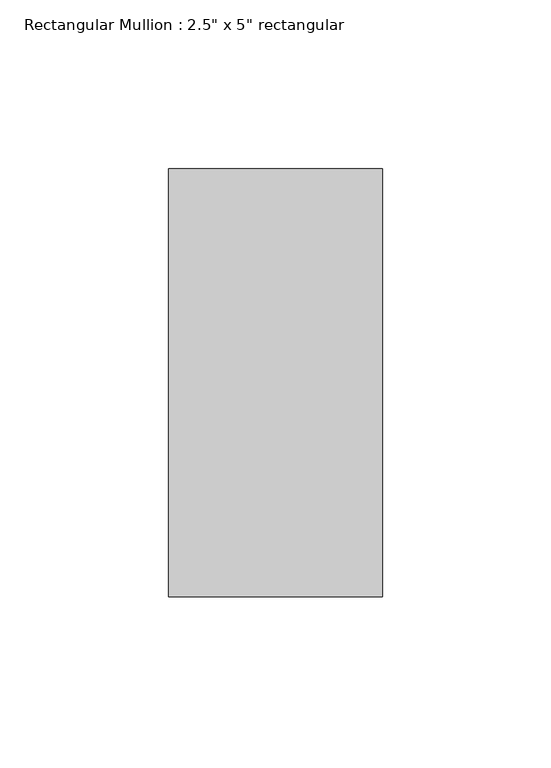
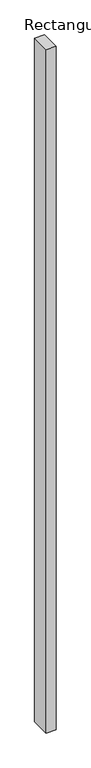
"""IFC4 building model written with IfcOpenShell, lengths in millimetres: member geometry."""

from ifc_helpers import new_model, si_unit, frame, origin, place, context, project, spatial, polyline, outline, extrude, source, transform, mapped, element, save


def member_44cf4dfe(model_context):
    return source(origin(), model_context, "Body", "SweptSolid", [
        extrude(outline(polyline([(0.0, 63.5), (0.0, -63.5), (-63.5, -63.5), (-63.5, 63.5), (0.0, 63.5)])), frame((0.0, 0.0, -4597.4), z_axis=(0.0, 0.0, 1.0), x_axis=(1.0, 0.0, 0.0)), (0.0, 0.0, 1.0), 4597.4),
    ])


if __name__ == "__main__":
    model = new_model("IFC4")
    model_context = context("Model", 3, world=origin())
    ifc_project = project(units=[si_unit("LENGTHUNIT", "METRE", prefix="MILLI")], contexts=[model_context])
    site = spatial("IfcSite", under=ifc_project)
    building = spatial("IfcBuilding", under=site)
    placement = place(None, origin())
    member_shape = member_44cf4dfe(model_context)
    element("IfcMember", 1, ObjectType="Rectangular Mullion : 2.5\" x 5\" rectangular", at=placement, inside=building, context=model_context, shape_type="MappedRepresentation", body=[
        mapped(member_shape, transform((0.0, 0.0, 0.0), x_axis=(1.0, 0.0, 0.0), y_axis=(0.0, 1.0, 0.0), z_axis=(0.0, 0.0, 1.0))),
    ])
    save(model, "model.ifc")

# Revit data of these elements
# Type "Rectangular Mullion : 2.5\" x 5\" rectangular"
#   built-in parameter 1007304 = 0.416667 (stored number, unit not read)
#   built-in parameter 1007301 = 0.104167 (stored number, unit not read)
#   built-in parameter 1007300 = 0.104167 (stored number, unit not read)
# Element 1 (IfcMember, "Rectangular Mullion : 2.5\" x 5\" rectangular")
#   Materials on its faces: "Aluminum"
# Materials
#   "Aluminum": class "Metal", colour RGB 247 247 247, transparency 0, Description = "Aluminum 6061", Cost = 0
